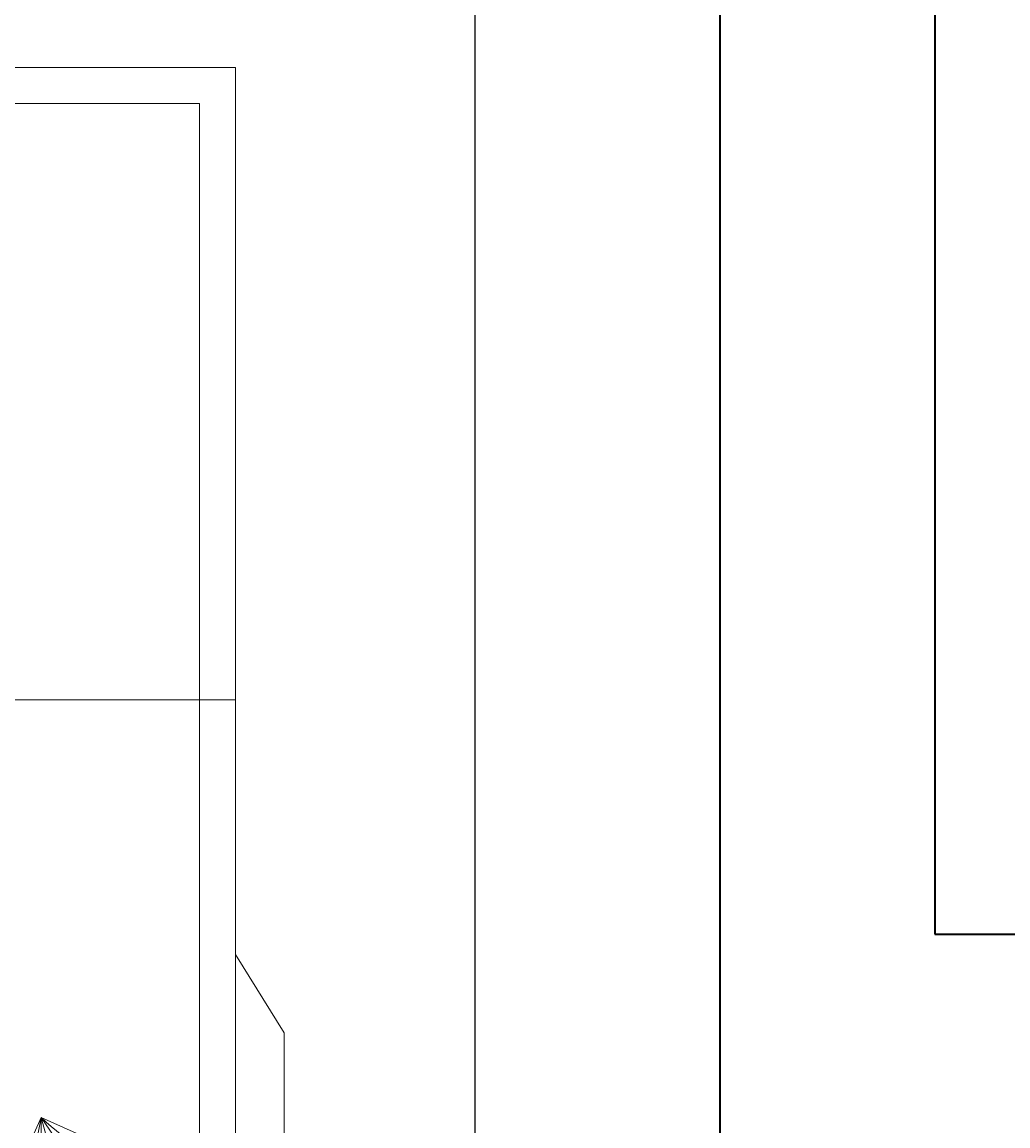
# Model space of a CAD drawing. Units: inches. Extents: x -61 to 1599, y -1316 to 257.
# Tile 83 of 204: x 240 to 268, y -373 to -342. Entities that reach past the tile are written whole.
import ezdxf

# ---------------------------------------------------------------- set-up
doc = ezdxf.new("R2010")
doc.units = ezdxf.units.IN
doc.header["$MEASUREMENT"] = 0
for name, color, linetype, lineweight in [('A-ANNO-DIMS', 2, 'Continuous', 18), ('FURNITURE', 83, 'Continuous', 18), ('WALLS', 4, 'Continuous', 35)]:
    doc.layers.add(name, color=color, linetype=linetype, lineweight=lineweight)
doc.styles.get("Standard").update_dxf_attribs({"font": 'arial.ttf'})
doc.dimstyles.get("Standard").update_dxf_attribs({"dimtxt": 0.18, "dimasz": 0.18, "dimexe": 0.18, "dimexo": 0.0625, "dimgap": 0.09, "dimtad": 0, "dimtih": 1, "dimtoh": 1, "dimdec": 0, "dimzin": 0, "dimdsep": 46, "dimlunit": 3, "dimtxsty": 'Standard', "dimcen": 0.09, "dimadec": 0, "dimazin": 0, "dimtfac": 1, "dimtdec": 0, "dimtofl": 0, "dimtmove": 0, "dimatfit": 3, "dimfxl": 1, "dimtolj": 1, "dimtzin": 0, "dimarcsym": 0})

# ---------------------------------------------------------------- blocks, each defined once
blk = doc.blocks.new('MASTER-BEDROOM-CONSOLE')
for p, q in [((0, 44.886), (23.587, 44.886)), ((23.587, 37.779), (23.587, 9.438)), ((23.587, 37.779), (24.943, 35.589)), ((24.943, 35.589), (24.943, 9.456)), ((18.162, 33.228), (18.879, 30.704)), ((18.162, 33.228), (19.133, 31.826)), ((18.162, 33.228), (18.181, 31.167)), ((23.587, 30.804), (21.228, 29.654)), ((23.587, 30.804), (21.894, 30.592)), ((23.587, 30.804), (22.038, 29.443)), ((18.441, 28.869), (18.678, 29.228)), ((19.963, 28.553), (19.841, 28.966)), ((18.203, 28.51), (18.441, 28.869)), ((20.085, 28.141), (19.963, 28.553)), ((19.008, 27.84), (18.886, 28.253)), ((19.184, 28.233), (19.008, 27.84)), ((19.309, 28.148), (19.008, 27.84)), ((19.008, 27.84), (18.615, 28.016)), ((19.008, 27.84), (18.707, 27.533)), ((19.008, 27.84), (18.833, 27.448)), ((19.401, 27.665), (19.008, 27.84)), ((19.13, 27.428), (19.008, 27.84)), ((18.061, 27.072), (17.939, 27.485)), ((19.618, 26.876), (19.855, 27.235)), ((18.183, 26.66), (18.061, 27.072)), ((19.38, 26.517), (19.618, 26.876)), ((18.084, 26.588), (18.801, 24.064)), ((18.084, 26.588), (19.055, 25.186)), ((18.084, 26.588), (18.103, 24.527)), ((14.429, 24.877), (15.978, 26.238)), ((14.429, 24.877), (16.788, 26.026)), ((14.429, 24.877), (16.122, 25.089)), ((19.854, 22.452), (19.137, 24.976)), ((19.854, 22.452), (19.835, 24.514)), ((23.509, 24.163), (21.15, 23.014)), ((23.509, 24.163), (21.816, 23.952)), ((23.509, 24.163), (21.96, 22.803)), ((19.854, 22.452), (18.883, 23.854)), ((0, 22.886), (23.587, 22.886)), ((18.362, 22.229), (18.6, 22.588)), ((18.125, 21.87), (18.362, 22.229)), ((19.885, 21.913), (19.763, 22.326)), ((20.007, 21.5), (19.885, 21.913)), ((18.93, 21.2), (18.808, 21.613)), ((19.105, 21.593), (18.93, 21.2)), ((18.93, 21.2), (18.537, 21.376)), ((19.23, 21.508), (18.93, 21.2)), ((18.93, 21.2), (18.629, 20.893)), ((18.93, 21.2), (18.754, 20.808)), ((19.322, 21.025), (18.93, 21.2)), ((19.052, 20.788), (18.93, 21.2)), ((17.983, 20.432), (17.861, 20.845)), ((18.105, 20.02), (17.983, 20.432)), ((19.54, 20.236), (19.777, 20.595)), ((19.302, 19.877), (19.54, 20.236)), ((18.084, 19.819), (18.801, 17.295)), ((18.084, 19.819), (19.055, 18.417)), ((18.084, 19.819), (18.103, 17.757)), ((14.351, 18.237), (15.9, 19.598)), ((14.351, 18.237), (16.71, 19.386)), ((14.351, 18.237), (16.043, 18.448)), ((19.776, 15.812), (19.059, 18.336)), ((19.776, 15.812), (19.757, 17.874)), ((23.509, 17.394), (21.15, 16.245)), ((23.509, 17.394), (21.816, 17.183)), ((23.509, 17.394), (21.96, 16.033)), ((19.776, 15.812), (18.804, 17.214)), ((18.362, 15.459), (18.6, 15.818)), ((18.125, 15.101), (18.362, 15.459)), ((19.885, 15.143), (19.763, 15.556)), ((20.007, 14.731), (19.885, 15.143)), ((18.93, 14.431), (18.808, 14.843)), ((19.105, 14.823), (18.93, 14.431)), ((18.93, 14.431), (18.537, 14.606)), ((19.23, 14.738), (18.93, 14.431)), ((18.93, 14.431), (18.629, 14.123)), ((18.93, 14.431), (18.754, 14.038)), ((19.322, 14.255), (18.93, 14.431)), ((19.052, 14.018), (18.93, 14.431)), ((17.983, 13.663), (17.861, 14.075)), ((18.105, 13.25), (17.983, 13.663)), ((19.54, 13.466), (19.777, 13.825)), ((19.302, 13.108), (19.54, 13.466)), ((14.351, 11.468), (15.9, 12.828)), ((14.351, 11.468), (16.71, 12.617)), ((14.351, 11.468), (16.043, 11.679)), ((19.776, 9.043), (19.059, 11.567)), ((19.776, 9.043), (19.757, 11.104)), ((19.776, 9.043), (18.804, 10.445)), ((22.587, 9.438), (23.587, 9.438)), ((1, 3.748), (0, 3.748))]:
    blk.add_line(p, q)
for points in [[(0, 3.748), (0, 62.524), (23.587, 62.524), (23.587, 9.438)], [(1, 3.748), (1, 61.524), (22.587, 61.524), (22.587, 9.438)]]:
    blk.add_lwpolyline(points)
for points in [[(14.429, 24.877), (18.162, 33.228), (23.587, 30.804), (19.854, 22.452)], [(14.351, 18.237), (18.084, 26.588), (23.509, 24.163), (19.776, 15.812)], [(14.351, 11.468), (18.084, 19.819), (23.509, 17.394), (19.776, 9.043)]]:
    blk.add_lwpolyline(points, close=True)
for centre, radius in [((19.008, 27.84), 0.567), ((19.008, 27.84), 0.567), ((19.008, 27.84), 0.43), ((18.93, 21.2), 0.567), ((18.93, 21.2), 0.567), ((18.93, 21.2), 0.43), ((18.93, 14.431), 0.567), ((18.93, 14.431), 0.567), ((18.93, 14.431), 0.43)]:
    blk.add_circle(centre, radius)
for centre, radius, start, end in [((0.46, 36.131), 17.938, 321.1446, 350.6879), ((24.495, 40.115), 9.356, 227.4013, 264.4312), ((19.167, 31.62), 0.209, 99.3213, 167.2974), ((18.925, 31.877), 0.214, 280.2125, 346.4062), ((19.095, 32.037), 0.214, 280.2125, 346.4062), ((19.338, 31.78), 0.209, 99.3213, 167.2974), ((18.215, 30.96), 0.209, 99.3213, 167.2974), ((17.973, 31.217), 0.214, 280.2125, 346.4062), ((18.143, 31.378), 0.214, 280.2125, 346.4062), ((18.385, 31.121), 0.209, 99.3213, 167.2974), ((18.841, 30.915), 0.214, 280.2125, 346.4062), ((19.083, 30.658), 0.209, 99.3213, 167.2974), ((37.556, 19.55), 17.938, 141.1446, 170.6879), ((22.077, 30.705), 0.214, 145.4264, 211.62), ((21.724, 30.714), 0.209, 324.5352, 32.5112), ((18.913, 30.498), 0.209, 99.3213, 167.2974), ((18.67, 30.755), 0.214, 280.2125, 346.4062), ((22.071, 30.471), 0.214, 145.4264, 211.62), ((21.718, 30.48), 0.209, 324.5352, 32.5112), ((21.411, 29.767), 0.214, 145.4264, 211.62), ((21.058, 29.776), 0.209, 324.5352, 32.5112), ((21.405, 29.533), 0.214, 145.4264, 211.62), ((21.052, 29.542), 0.209, 324.5352, 32.5112), ((22.221, 29.555), 0.214, 145.4264, 211.62), ((21.867, 29.564), 0.209, 324.5352, 32.5112), ((22.215, 29.321), 0.214, 145.4264, 211.62), ((21.861, 29.33), 0.209, 324.5352, 32.5112), ((0.382, 29.491), 17.938, 321.1446, 350.6879), ((24.416, 33.475), 9.356, 227.4013, 264.4312), ((16.149, 26.117), 0.209, 144.5352, 212.5112), ((16.155, 26.351), 0.209, 144.5352, 212.5112), ((15.796, 26.126), 0.214, 325.4264, 31.62), ((15.802, 26.36), 0.214, 325.4264, 31.62), ((16.965, 26.139), 0.209, 144.5352, 212.5112), ((16.611, 26.148), 0.214, 325.4264, 31.62), ((16.959, 25.905), 0.209, 144.5352, 212.5112), ((16.605, 25.914), 0.214, 325.4264, 31.62), ((16.298, 25.201), 0.209, 144.5352, 212.5112), ((15.945, 25.21), 0.214, 325.4264, 31.62), ((19.017, 25.397), 0.214, 280.2125, 346.4062), ((19.259, 25.14), 0.209, 99.3213, 167.2974), ((16.292, 24.967), 0.209, 144.5352, 212.5112), ((15.939, 24.976), 0.214, 325.4264, 31.62), ((19.089, 24.98), 0.209, 99.3213, 167.2974), ((18.847, 25.237), 0.214, 280.2125, 346.4062), ((19.175, 24.765), 0.214, 100.2125, 166.4062), ((18.933, 25.022), 0.209, 279.3213, 347.2974), ((19.103, 25.183), 0.209, 279.3213, 347.2974), ((19.346, 24.926), 0.214, 100.2125, 166.4062), ((13.521, 15.565), 9.356, 47.4013, 84.4312), ((18.065, 24.738), 0.214, 280.2125, 346.4062), ((18.307, 24.48), 0.209, 99.3213, 167.2974), ((19.801, 24.721), 0.209, 279.3213, 347.2974), ((20.043, 24.464), 0.214, 100.2125, 166.4062), ((18.137, 24.32), 0.209, 99.3213, 167.2974), ((17.894, 24.577), 0.214, 280.2125, 346.4062), ((19.873, 24.303), 0.214, 100.2125, 166.4062), ((19.631, 24.56), 0.209, 279.3213, 347.2974), ((18.834, 23.858), 0.209, 99.3213, 167.2974), ((18.592, 24.115), 0.214, 280.2125, 346.4062), ((18.763, 24.275), 0.214, 280.2125, 346.4062), ((19.005, 24.018), 0.209, 99.3213, 167.2974), ((37.478, 12.91), 17.938, 141.1446, 170.6879), ((21.999, 24.065), 0.214, 145.4264, 211.62), ((21.646, 24.074), 0.209, 324.5352, 32.5112), ((18.921, 23.643), 0.214, 100.2125, 166.4062), ((18.678, 23.9), 0.209, 279.3213, 347.2974), ((18.849, 24.061), 0.209, 279.3213, 347.2974), ((19.091, 23.804), 0.214, 100.2125, 166.4062), ((21.993, 23.83), 0.214, 145.4264, 211.62), ((21.64, 23.84), 0.209, 324.5352, 32.5112), ((21.332, 23.127), 0.214, 145.4264, 211.62), ((20.979, 23.136), 0.209, 324.5352, 32.5112), ((21.326, 22.892), 0.214, 145.4264, 211.62), ((20.973, 22.902), 0.209, 324.5352, 32.5112), ((22.136, 22.681), 0.214, 145.4264, 211.62), ((22.142, 22.915), 0.214, 145.4264, 211.62), ((21.783, 22.69), 0.209, 324.5352, 32.5112), ((21.789, 22.924), 0.209, 324.5352, 32.5112), ((0.382, 22.721), 17.938, 321.1446, 350.6879), ((16.076, 19.711), 0.209, 144.5352, 212.5112), ((15.723, 19.72), 0.214, 325.4264, 31.62), ((24.416, 26.706), 9.356, 227.4013, 264.4312), ((16.07, 19.476), 0.209, 144.5352, 212.5112), ((15.717, 19.486), 0.214, 325.4264, 31.62), ((16.886, 19.499), 0.209, 144.5352, 212.5112), ((16.533, 19.508), 0.214, 325.4264, 31.62), ((16.88, 19.265), 0.209, 144.5352, 212.5112), ((16.527, 19.274), 0.214, 325.4264, 31.62), ((16.22, 18.561), 0.209, 144.5352, 212.5112), ((15.867, 18.57), 0.214, 325.4264, 31.62), ((19.017, 18.628), 0.214, 280.2125, 346.4062), ((19.259, 18.371), 0.209, 99.3213, 167.2974), ((19.025, 18.543), 0.209, 279.3213, 347.2974), ((19.267, 18.286), 0.214, 100.2125, 166.4062), ((13.443, 8.925), 9.356, 47.4013, 84.4312), ((16.214, 18.327), 0.209, 144.5352, 212.5112), ((15.861, 18.336), 0.214, 325.4264, 31.62), ((19.089, 18.21), 0.209, 99.3213, 167.2974), ((18.847, 18.467), 0.214, 280.2125, 346.4062), ((19.097, 18.125), 0.214, 100.2125, 166.4062), ((18.855, 18.382), 0.209, 279.3213, 347.2974), ((18.065, 17.968), 0.214, 280.2125, 346.4062), ((18.307, 17.711), 0.209, 99.3213, 167.2974), ((19.795, 17.663), 0.214, 100.2125, 166.4062), ((19.552, 17.92), 0.209, 279.3213, 347.2974), ((19.723, 18.081), 0.209, 279.3213, 347.2974), ((19.965, 17.824), 0.214, 100.2125, 166.4062), ((18.137, 17.55), 0.209, 99.3213, 167.2974), ((17.894, 17.807), 0.214, 280.2125, 346.4062), ((18.834, 17.088), 0.209, 99.3213, 167.2974), ((18.592, 17.345), 0.214, 280.2125, 346.4062), ((18.763, 17.506), 0.214, 280.2125, 346.4062), ((19.005, 17.249), 0.209, 99.3213, 167.2974), ((18.771, 17.421), 0.209, 279.3213, 347.2974), ((19.013, 17.164), 0.214, 100.2125, 166.4062), ((37.478, 6.14), 17.938, 141.1446, 170.6879), ((21.999, 17.295), 0.214, 145.4264, 211.62), ((21.646, 17.304), 0.209, 324.5352, 32.5112), ((18.842, 17.003), 0.214, 100.2125, 166.4062), ((18.6, 17.26), 0.209, 279.3213, 347.2974), ((21.993, 17.061), 0.214, 145.4264, 211.62), ((21.64, 17.07), 0.209, 324.5352, 32.5112), ((21.332, 16.357), 0.214, 145.4264, 211.62), ((20.979, 16.366), 0.209, 324.5352, 32.5112), ((21.326, 16.123), 0.214, 145.4264, 211.62), ((20.973, 16.132), 0.209, 324.5352, 32.5112), ((22.136, 15.911), 0.214, 145.4264, 211.62), ((22.142, 16.145), 0.214, 145.4264, 211.62), ((21.783, 15.92), 0.209, 324.5352, 32.5112), ((21.789, 16.155), 0.209, 324.5352, 32.5112), ((16.076, 12.941), 0.209, 144.5352, 212.5112), ((15.723, 12.95), 0.214, 325.4264, 31.62), ((16.07, 12.707), 0.209, 144.5352, 212.5112), ((15.717, 12.716), 0.214, 325.4264, 31.62), ((16.886, 12.729), 0.209, 144.5352, 212.5112), ((16.533, 12.739), 0.214, 325.4264, 31.62), ((16.88, 12.495), 0.209, 144.5352, 212.5112), ((16.527, 12.504), 0.214, 325.4264, 31.62), ((16.22, 11.791), 0.209, 144.5352, 212.5112), ((15.867, 11.801), 0.214, 325.4264, 31.62), ((19.025, 11.773), 0.209, 279.3213, 347.2974), ((19.267, 11.516), 0.214, 100.2125, 166.4062), ((13.443, 2.156), 9.356, 47.4013, 84.4312), ((16.214, 11.557), 0.209, 144.5352, 212.5112), ((15.861, 11.566), 0.214, 325.4264, 31.62), ((19.097, 11.356), 0.214, 100.2125, 166.4062), ((18.855, 11.613), 0.209, 279.3213, 347.2974), ((19.795, 10.893), 0.214, 100.2125, 166.4062), ((19.552, 11.151), 0.209, 279.3213, 347.2974), ((19.723, 11.311), 0.209, 279.3213, 347.2974), ((19.965, 11.054), 0.214, 100.2125, 166.4062), ((18.771, 10.651), 0.209, 279.3213, 347.2974), ((19.013, 10.394), 0.214, 100.2125, 166.4062), ((18.842, 10.234), 0.214, 100.2125, 166.4062), ((18.6, 10.491), 0.209, 279.3213, 347.2974), ((10.308, 16.053), 16.053, 230.0449, 335.7344), ((9.449, 17.042), 16.053, 233.9382, 331.7264)]:
    blk.add_arc(centre, radius, start, end)
for points in [[(18.203, 28.51), (18.191, 28.604), (18.167, 28.791), (18.438, 28.884), (18.778, 28.897), (18.67, 29.157), (18.678, 29.228)], [(20.085, 28.141), (20.124, 28.226), (20.202, 28.398), (19.97, 28.566), (19.649, 28.679), (19.829, 28.896), (19.841, 28.966)], [(19.309, 28.148), (19.303, 28.054), (19.292, 27.866), (19.008, 27.825), (18.671, 27.876), (18.729, 27.6), (18.707, 27.533)], [(19.13, 27.428), (19.169, 27.514), (19.247, 27.685), (19.015, 27.854), (18.694, 27.966), (18.873, 28.183), (18.886, 28.253)], [(19.184, 28.233), (19.098, 28.193), (18.927, 28.113), (18.994, 27.835), (19.165, 27.54), (18.888, 27.492), (18.833, 27.448)], [(19.401, 27.665), (19.361, 27.75), (19.281, 27.921), (19.003, 27.854), (18.708, 27.683), (18.66, 27.961), (18.615, 28.016)], [(18.183, 26.66), (18.222, 26.746), (18.3, 26.917), (18.069, 27.086), (17.747, 27.198), (17.927, 27.415), (17.939, 27.485)], [(19.38, 26.517), (19.368, 26.611), (19.344, 26.798), (19.615, 26.891), (19.955, 26.904), (19.847, 27.164), (19.855, 27.235)], [(18.125, 21.87), (18.113, 21.964), (18.089, 22.151), (18.359, 22.244), (18.7, 22.257), (18.592, 22.517), (18.6, 22.588)], [(20.007, 21.5), (20.046, 21.586), (20.124, 21.758), (19.892, 21.926), (19.571, 22.039), (19.75, 22.256), (19.763, 22.326)], [(19.052, 20.788), (19.091, 20.874), (19.169, 21.045), (18.937, 21.214), (18.615, 21.326), (18.795, 21.543), (18.808, 21.613)], [(19.105, 21.593), (19.02, 21.553), (18.849, 21.473), (18.916, 21.195), (19.087, 20.9), (18.809, 20.852), (18.754, 20.808)], [(19.322, 21.025), (19.283, 21.11), (19.203, 21.281), (18.924, 21.214), (18.63, 21.043), (18.582, 21.321), (18.537, 21.376)], [(19.23, 21.508), (19.225, 21.414), (19.213, 21.226), (18.93, 21.185), (18.593, 21.236), (18.651, 20.96), (18.629, 20.893)], [(18.105, 20.02), (18.144, 20.105), (18.222, 20.277), (17.99, 20.445), (17.669, 20.558), (17.848, 20.775), (17.861, 20.845)], [(19.302, 19.877), (19.29, 19.971), (19.266, 20.158), (19.537, 20.251), (19.877, 20.264), (19.769, 20.524), (19.777, 20.595)], [(18.125, 15.101), (18.113, 15.194), (18.089, 15.381), (18.359, 15.474), (18.7, 15.488), (18.592, 15.748), (18.6, 15.818)], [(20.007, 14.731), (20.046, 14.817), (20.124, 14.988), (19.892, 15.157), (19.571, 15.269), (19.75, 15.486), (19.763, 15.556)], [(19.052, 14.018), (19.091, 14.104), (19.169, 14.276), (18.937, 14.444), (18.615, 14.557), (18.795, 14.773), (18.808, 14.843)], [(19.105, 14.823), (19.02, 14.784), (18.849, 14.704), (18.916, 14.425), (19.087, 14.131), (18.809, 14.083), (18.754, 14.038)], [(19.322, 14.255), (19.283, 14.341), (19.203, 14.511), (18.924, 14.445), (18.63, 14.274), (18.582, 14.551), (18.537, 14.606)], [(19.23, 14.738), (19.225, 14.644), (19.213, 14.456), (18.93, 14.416), (18.593, 14.466), (18.651, 14.191), (18.629, 14.123)], [(18.105, 13.25), (18.144, 13.336), (18.222, 13.508), (17.99, 13.676), (17.669, 13.788), (17.848, 14.005), (17.861, 14.075)], [(19.302, 13.108), (19.29, 13.201), (19.266, 13.388), (19.537, 13.481), (19.877, 13.495), (19.769, 13.755), (19.777, 13.825)]]:
    blk.add_open_spline(points, degree=3, knots=[0, 0, 0, 0, 0.249187, 0.498374, 0.766554, 1.034734, 1.034734, 1.034734, 1.034734])
blk = doc.blocks.new('*D687')
at = {"layer": 'A-ANNO-DIMS', "color": 0, "lineweight": -2, "transparency": 16777216}
for p, q in [((289.418, 181.677), (-61.077, 181.677)), ((-60.897, 181.497), (-60.897, -528.952)), ((-60.897, -1239.765), (-60.897, -529.316)), ((319.64, -1239.945), (-61.077, -1239.945))]:
    blk.add_line(p, q, dxfattribs=at)
at = {"layer": 'A-ANNO-DIMS', "color": 0, "transparency": 16777216}
for points in [[(-60.927, 181.497), (-60.867, 181.497), (-60.897, 181.677)], [(-60.927, -1239.765), (-60.867, -1239.765), (-60.897, -1239.945)]]:
    blk.add_solid(points, dxfattribs=at)
at = {"layer": 'DEFPOINTS', "color": 0, "transparency": 16777216}
for p in [(289.481, 181.677), (-60.897, -1239.945), (319.703, -1239.945)]:
    blk.add_point(p, dxfattribs=at)
at = {"layer": 'A-ANNO-DIMS', "color": 0, "transparency": 16777216, "insert": (-60.897, -529.134), "char_height": 0.18, "attachment_point": 5}
blk.add_mtext('\\A1;1421.6', dxfattribs=at)
blk = doc.blocks.new('*D699')
at = {"layer": 'A-ANNO-DIMS', "color": 0, "lineweight": -2, "transparency": 16777216}
for p, q in [((835.64, -167.169), (-61.077, -167.169)), ((-60.897, -167.349), (-60.897, -306.726)), ((-60.897, -446.466), (-60.897, -307.09)), ((841.64, -446.646), (-61.077, -446.646))]:
    blk.add_line(p, q, dxfattribs=at)
at = {"layer": 'A-ANNO-DIMS', "color": 0, "transparency": 16777216}
for points in [[(-60.927, -167.349), (-60.867, -167.349), (-60.897, -167.169)], [(-60.927, -446.466), (-60.867, -446.466), (-60.897, -446.646)]]:
    blk.add_solid(points, dxfattribs=at)
at = {"layer": 'DEFPOINTS', "color": 0, "transparency": 16777216}
for p in [(835.703, -167.169), (-60.897, -446.646), (841.703, -446.646)]:
    blk.add_point(p, dxfattribs=at)
at = {"layer": 'A-ANNO-DIMS', "color": 0, "transparency": 16777216, "insert": (-60.897, -306.908), "char_height": 0.18, "attachment_point": 5}
blk.add_mtext('\\A1;279.5', dxfattribs=at)
blk = doc.blocks.new('*D701')
at = {"layer": 'A-ANNO-DIMS', "color": 0, "lineweight": -2, "transparency": 16777216}
for p, q in [((215.752, -616.882), (215.752, 257.457)), ((215.932, 257.277), (233.924, 257.277)), ((252.702, 257.277), (234.711, 257.277)), ((252.882, -616.882), (252.882, 257.457))]:
    blk.add_line(p, q, dxfattribs=at)
at = {"layer": 'A-ANNO-DIMS', "color": 0, "transparency": 16777216}
for points in [[(215.932, 257.307), (215.932, 257.247), (215.752, 257.277)], [(252.702, 257.307), (252.702, 257.247), (252.882, 257.277)]]:
    blk.add_solid(points, dxfattribs=at)
at = {"layer": 'DEFPOINTS', "color": 0, "transparency": 16777216}
for p in [(252.882, 257.277), (215.752, -616.945), (252.882, -616.945)]:
    blk.add_point(p, dxfattribs=at)
at = {"layer": 'A-ANNO-DIMS', "color": 0, "transparency": 16777216, "insert": (234.317, 257.277), "char_height": 0.18, "attachment_point": 5}
blk.add_mtext('\\A1;37.13', dxfattribs=at)

msp = doc.modelspace()

# ---------------------------------------------------------------- linework, layer by layer
at = {"layer": 'WALLS'}
for p, q in [((259.7028, -288.3229), (259.7028, -432.3229)), ((265.7028, -288.3229), (265.7028, -367.3229)), ((265.7028, -367.3229), (319.7028, -367.3229))]:
    msp.add_line(p, q, dxfattribs=at)

# ---------------------------------------------------------------- block references
at = {"layer": 'FURNITURE'}
msp.add_blockref('MASTER-BEDROOM-CONSOLE', (222.602, -405.667), dxfattribs=at)

# ---------------------------------------------------------------- dimensions: what is measured, and where the dimension line sits
at = {"layer": 'A-ANNO-DIMS'}
dim = msp.add_linear_dim(base=(252.8825, 257.2771), p1=(215.7521, -616.9446), p2=(252.8825, -616.9446), dimstyle='Standard', override={"dimdec": 2, "dimlfac": 1, "dimrnd": 0, "dimzin": 0, "dimdsep": 46, "dimlunit": 2}, dxfattribs=at)
dim.commit()
dim.dimension.update_dxf_attribs({"geometry": '*D701', "text_midpoint": (234.3173, 257.2771)})
for base, p1, p2, picture, middle in [((-60.8972, -1239.9446), (289.4807, 181.6771), (319.7028, -1239.9446), '*D687', (-60.8972, -529.1337)), ((-60.8972, -446.6462), (835.7028, -167.169), (841.7028, -446.6462), '*D699', (-60.8972, -306.9076))]:
    dim = msp.add_linear_dim(base=base, p1=p1, p2=p2, angle=90, dimstyle='Standard', override={"dimdec": 1, "dimlfac": 1, "dimrnd": 0, "dimzin": 0, "dimdsep": 46, "dimlunit": 2}, dxfattribs=at)
    dim.commit()
    dim.dimension.update_dxf_attribs({"geometry": picture, "text_midpoint": middle})

doc.saveas('drawing.dxf')
